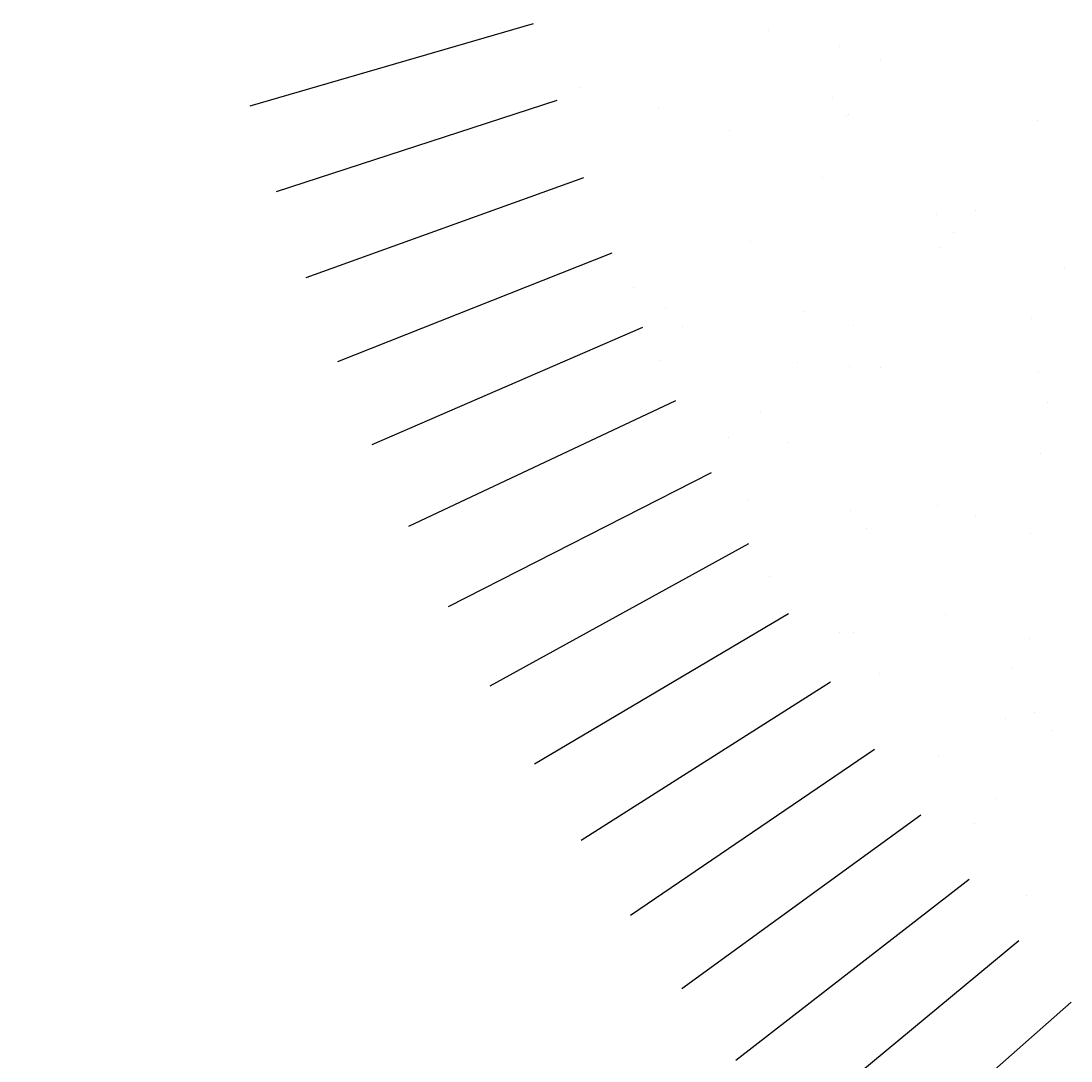
# Model space of a CAD drawing. Units: millimetres. Extents: x -857 to 54106, y -13666 to 13947.
# Tile 30 of 41: x 30856 to 31338, y 8975 to 9453. Entities that reach past the tile are written whole.
import ezdxf

# ---------------------------------------------------------------- set-up
doc = ezdxf.new("R2010")
doc.units = ezdxf.units.MM
doc.layers.add('A-ANNO-DIMS', color=2, linetype='Continuous', lineweight=18)
doc.layers.add('A-FURN', color=21, linetype='Continuous', lineweight=18)
doc.layers.add('A-HT', color=15, linetype='Continuous')
doc.styles.get("Standard").update_dxf_attribs({"font": 'arial.ttf'})
doc.dimstyles.new('ISO-25', dxfattribs={"dimtxt": 2.5, "dimasz": 2.5, "dimexe": 1.25, "dimexo": 0.625, "dimtad": 1, "dimtxsty": 'Standard', "dimcen": 2.5, "dimadec": 0, "dimazin": 0, "dimtfac": 1, "dimtmove": 0, "dimatfit": 3, "dimfxl": 1, "dimarcsym": 0})

# ---------------------------------------------------------------- blocks, each defined once
blk = doc.blocks.new('*X18')
at = {"color": 0}
for p, q in [((2.39488, 2.77498), (2.39488, 2.77498)), ((2.49675, 2.7473), (2.49675, 2.7473)), ((2.40566, 2.73475), (2.40566, 2.73475)), ((2.53357, 2.73414), (2.53357, 2.73414)), ((2.50737, 2.73126), (2.50737, 2.73126)), ((2.51659, 2.72281), (2.51659, 2.72281)), ((2.41695, 2.69867), (2.41695, 2.69867)), ((2.57265, 2.69895), (2.57265, 2.69895)), ((2.60415, 2.68954), (2.60415, 2.68954)), ((2.47327, 2.68787), (2.47327, 2.68787)), ((2.36628, 2.67893), (2.36628, 2.67893)), ((2.56009, 2.68295), (2.56009, 2.68295)), ((2.64348, 2.67826), (2.64348, 2.67826)), ((2.57557, 2.66932), (2.57557, 2.66932)), ((2.53492, 2.66396), (2.53492, 2.66396)), ((2.50889, 2.66054), (2.50889, 2.66054)), ((2.44098, 2.6516), (2.44098, 2.6516)), ((2.37431, 2.64282), (2.37431, 2.64282)), ((2.40033, 2.64625), (2.40033, 2.64625)), ((2.67176, 2.64266), (2.67176, 2.64266)), ((2.40881, 2.63841), (2.40881, 2.63841)), ((2.40978, 2.63907), (2.40978, 2.63907)), ((2.53672, 2.6378), (2.53672, 2.6378)), ((2.60985, 2.63735), (2.60985, 2.63735)), ((2.51605, 2.63553), (2.51605, 2.63553)), ((2.67175, 2.63582), (2.67175, 2.63582)), ((2.61907, 2.62891), (2.61907, 2.62891)), ((2.38142, 2.62182), (2.38142, 2.62182)), ((2.53713, 2.6221), (2.53713, 2.6221)), ((2.69284, 2.62238), (2.69284, 2.62238)), ((2.45955, 2.59347), (2.45955, 2.59347)), ((2.6073, 2.5932), (2.6073, 2.5932)), ((2.47642, 2.59153), (2.47642, 2.59153)), ((2.66257, 2.58905), (2.66257, 2.58905)), ((2.7352, 2.59259), (2.7352, 2.59259)), ((2.46876, 2.58502), (2.46876, 2.58502)), ((2.45733, 2.57346), (2.45733, 2.57346)), ((2.61304, 2.57374), (2.61304, 2.57374)), ((2.76874, 2.57403), (2.76874, 2.57403)), ((2.75626, 2.56365), (2.75626, 2.56365)), ((2.71561, 2.55829), (2.71561, 2.55829)), ((2.68958, 2.55487), (2.68958, 2.55487)), ((2.51226, 2.54516), (2.51226, 2.54516)), ((2.62167, 2.54593), (2.62167, 2.54593)), ((2.67491, 2.54632), (2.67491, 2.54632)), ((2.80579, 2.54799), (2.80579, 2.54799)), ((2.41196, 2.54207), (2.41196, 2.54207)), ((2.53986, 2.54145), (2.53986, 2.54145)), ((2.58102, 2.54058), (2.58102, 2.54058)), ((2.71234, 2.54344), (2.71234, 2.54344)), ((2.55499, 2.53715), (2.55499, 2.53715)), ((2.72155, 2.535), (2.72155, 2.535)), ((2.48708, 2.52821), (2.48708, 2.52821))]:
    blk.add_line(p, q, dxfattribs=at)
blk = doc.blocks.new('A$C6796526C')
at = {"layer": 'A-HT'}
for p, q in [((2.30971, 0.47486), (2.4089, 0.36234)), ((2.27865, 0.44833), (2.37427, 0.33276)), ((2.24744, 0.42304), (2.33938, 0.30451)), ((2.21479, 0.39852), (2.30295, 0.27716)), ((2.18137, 0.37503), (2.26569, 0.25097)), ((2.14724, 0.35261), (2.22761, 0.22596)), ((2.11242, 0.33127), (2.18877, 0.20216)), ((2.07694, 0.31104), (2.14921, 0.17959)), ((2.04085, 0.29193), (2.10895, 0.15828)), ((2.00418, 0.27396), (2.06804, 0.13824)), ((1.96696, 0.25716), (2.02653, 0.1195)), ((1.92923, 0.24153), (1.98445, 0.10206)), ((1.89102, 0.22709), (1.94183, 0.08596)), ((1.85172, 0.21363), (1.89807, 0.07097)), ((1.81269, 0.20162), (1.85454, 0.05757))]:
    blk.add_line(p, q, dxfattribs=at)
at = {"layer": 'A-HT', "extrusion": (0, 0, -1), "zscale": -1, "rotation": 180}
blk.add_blockref('*X18', (0.55, 3), dxfattribs=at)
blk = doc.blocks.new('*D48')
at = {"layer": 'A-ANNO-DIMS', "color": 0, "lineweight": -2, "transparency": 16777216}
for p, q in [((30908.63, 11089.46), (30501.38, 11089.46)), ((30502.63, 11086.96), (30502.63, 8471.5)), ((30908.63, 8469), (30501.38, 8469))]:
    blk.add_line(p, q, dxfattribs=at)
at = {"layer": 'A-ANNO-DIMS', "color": 0, "transparency": 16777216}
for points in [[(30502.21, 11086.96), (30503.05, 11086.96), (30502.63, 11089.46)], [(30502.21, 8471.5), (30503.05, 8471.5), (30502.63, 8469)]]:
    blk.add_solid(points, dxfattribs=at)
at = {"layer": 'Defpoints', "color": 0, "transparency": 16777216}
for p in [(30909.25, 11089.46), (30502.63, 8469), (30909.25, 8469)]:
    blk.add_point(p, dxfattribs=at)
at = {"layer": 'A-ANNO-DIMS', "color": 0, "transparency": 16777216, "insert": (30500.73, 9779.23), "char_height": 2.5, "attachment_point": 5, "rotation": 90}
blk.add_mtext('2620 TYP.', dxfattribs=at)

msp = doc.modelspace()

# ---------------------------------------------------------------- block references
at = {"layer": 'A-FURN', "xscale": 903.6084929786902, "yscale": 903.6084929786902, "zscale": 903.6084929786902, "rotation": 269.9999999999988}
msp.add_blockref('A$C6796526C', (30909.253, 11089.463), dxfattribs=at)

# ---------------------------------------------------------------- dimensions: what is measured, and where the dimension line sits
at = {"layer": 'A-ANNO-DIMS'}
dim = msp.add_linear_dim(base=(30502.63, 8468.999), p1=(30909.254, 11089.463), p2=(30909.254, 8468.999), angle=270, text='<> TYP.', dimstyle='ISO-25', override={"dimdec": 0, "dimrnd": 0, "dimzin": 0, "dimlunit": 2}, dxfattribs=at)
dim.commit()
dim.dimension.update_dxf_attribs({"geometry": '*D48', "text_midpoint": (30500.728, 9779.231)})

doc.saveas('drawing.dxf')
